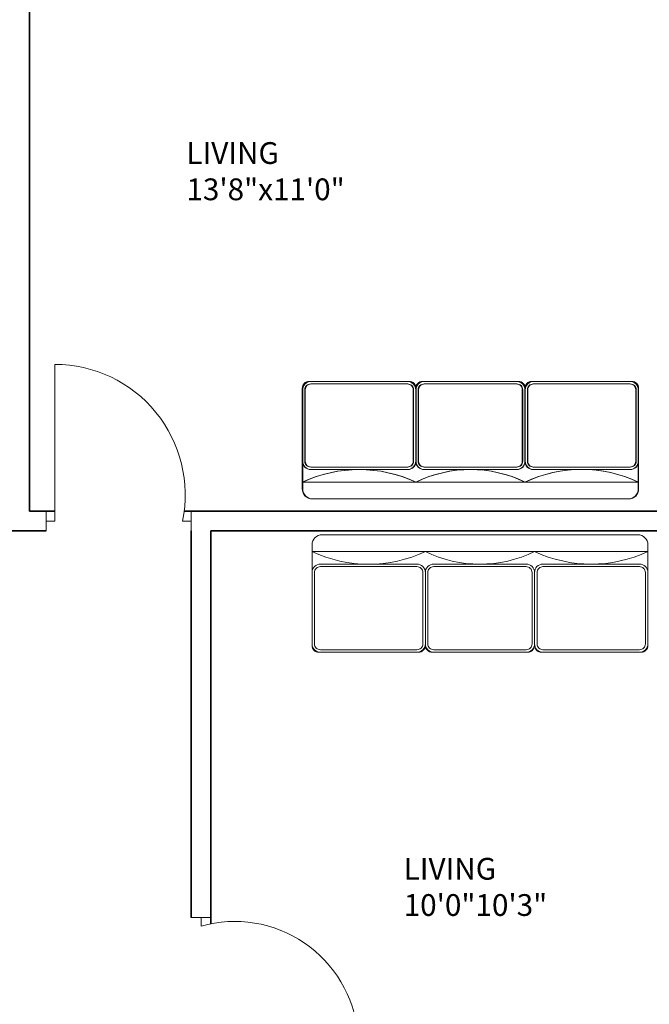
# Model space of a CAD drawing. Units: inches. Extents: x 2234 to 3001, y 1541 to 2386.
# Tile 8 of 12: x 2599 to 2744, y 1891 to 2118. Entities that reach past the tile are written whole.
import ezdxf

# ---------------------------------------------------------------- set-up
doc = ezdxf.new("R2010")
doc.units = ezdxf.units.IN
for name, color, linetype, lineweight in [('A-AREA-IDEN', 7, 'Continuous', 18), ('A-DOOR', 3, 'Continuous', 18), ('A-FURN', 9, 'Continuous', 13), ('A-WALL', 7, 'Continuous', 35)]:
    doc.layers.add(name, color=color, linetype=linetype, lineweight=lineweight)
doc.styles.get("Standard").update_dxf_attribs({"font": 'arial.ttf'})

# ---------------------------------------------------------------- blocks, each defined once
blk = doc.blocks.new('SOFA-3-SEAT')
for points in [[(1.93, 51.12), (18.33, 51.12, 0.414214), (20.26, 53.05), (20.26, 75.24, 0.414214), (18.33, 77.16), (1.93, 77.16, 0.414214), (0, 75.24), (0, 53.05, 0.414214)], [(1.93, 51.7), (18.33, 51.7, 0.414214), (19.68, 53.05), (19.68, 75.24, 0.414214), (18.33, 76.59), (1.93, 76.59, 0.414214), (0.58, 75.24), (0.58, 53.05, 0.414214)], [(1.93, 51.12), (18.33, 51.12, -0.414214), (20.26, 49.19), (20.26, 27.97, -0.414214), (18.33, 26.04), (1.93, 26.04, -0.414214), (0, 27.97), (0, 49.19, -0.414214)], [(1.93, 50.54), (18.33, 50.54, -0.414214), (19.68, 49.19), (19.68, 27.97, -0.414214), (18.33, 26.62), (1.93, 26.62, -0.414214), (0.58, 27.97), (0.58, 49.19, -0.414214)], [(1.93, 0), (18.33, 0, 0.414214), (20.26, 1.93), (20.26, 24.11, 0.414214), (18.33, 26.04), (1.93, 26.04, 0.414214), (0, 24.11), (0, 1.93, 0.414214)], [(1.93, 0.58), (18.33, 0.58, 0.414214), (19.68, 1.93), (19.68, 24.11, 0.414214), (18.33, 25.46), (1.93, 25.46, 0.414214), (0.58, 24.11), (0.58, 1.93, 0.414214)]]:
    blk.add_lwpolyline(points, format="xyb", close=True)
at = {"ltscale": 0.03}
blk.add_lwpolyline([(0, 24.48), (0, 1.54, 0.414214), (1.54, 0), (24.69, 0, 0.414214), (27.01, 2.31), (27.01, 74.85, 0.414214), (24.69, 77.16), (1.54, 77.16, 0.414214), (0, 75.62), (0, 52.68, 0.414214), (1.54, 51.14, -1), (1.54, 51.1, 0.414214), (0, 49.56), (0, 27.61, 0.414214), (1.54, 26.06, -1), (1.54, 26.02, 0.414214)], format="xyb", close=True, dxfattribs=at)
blk.add_lwpolyline([(23.15, 0), (23.15, 77.16)])
for centre, radius, start, end in [((50.64, 64.14), 30.42, 154.6538, 205.3462), ((48.71, 38.58), 28.47, 153.869, 206.131), ((50.96, 13.02), 30.71, 154.9106, 205.0894)]:
    blk.add_arc(centre, radius, start, end)

msp = doc.modelspace()

# ---------------------------------------------------------------- linework, layer by layer
at = {"layer": 'A-DOOR'}
for p, q in [((2607.0604, 2002.361), (2607.0604, 2038.361)), ((2605.0604, 2004.611), (2605.0604, 2000.111)), ((2638.4141, 2004.611), (2638.4141, 2004.611)), ((2638.4141, 2004.611), (2638.4141, 2000.111)), ((2605.0604, 2000.111), (2605.0604, 2002.361)), ((2605.0604, 2002.361), (2607.0604, 2002.361)), ((2638.4141, 2002.361), (2636.4141, 2002.361)), ((2638.4141, 2000.111), (2638.4141, 2002.361)), ((2638.4141, 1911.322), (2642.9141, 1911.322)), ((2642.9141, 1911.322), (2640.6641, 1911.322)), ((2640.6641, 1911.322), (2640.6641, 1909.322))]:
    msp.add_line(p, q, dxfattribs=at)
for centre, radius, start, end in [((2607.0604, 2008.3938), 29.9672, 348.38617, 90), ((2648.3788, 1881.9579), 28.4308, 5.798117, 105.744641)]:
    msp.add_arc(centre, radius, start, end, dxfattribs=at)
at = {"layer": 'A-WALL'}
for p, q in [((2601.2534, 2145.611), (2601.2534, 2004.611)), ((2601.2534, 2004.611), (2607.0604, 2004.611)), ((2636.7879, 2004.611), (2759.2534, 2004.611)), ((2593.6832, 2000.111), (2605.0604, 2000.111)), ((2638.4141, 2000.111), (2638.4141, 1911.322)), ((2642.9141, 2000.111), (2759.2534, 2000.111)), ((2642.9141, 2000.111), (2642.9141, 2000.111)), ((2642.9141, 1909.8586), (2642.9141, 2000.111))]:
    msp.add_line(p, q, dxfattribs=at)

# ---------------------------------------------------------------- block references
at = {"layer": 'A-FURN'}
for p, rotation in [((2663.9269, 2034.4483), 270), ((2663.9269, 2034.4483), 270), ((2664.0279, 2034.4483), 270), ((2664.0279, 2034.4483), 270), ((2743.3129, 1972.2215), 90), ((2743.3129, 1972.2215), 90)]:
    msp.add_blockref('SOFA-3-SEAT', p, dxfattribs=dict(at, rotation=rotation))

# ---------------------------------------------------------------- texts
at = {"layer": 'A-AREA-IDEN', "char_height": 5, "attachment_point": 1}
for s, width, insert in [('LIVING\\P13\'8"x11\'0"', 102.763163, (2637.303, 2089.4016)), ('LIVING\\P10\'0"10\'3"', 237.459688, (2687.2139, 1924.9979))]:
    msp.add_mtext_dynamic_manual_height_columns(s, width=width, gutter_width=12.5, heights=[0], dxfattribs=dict(at, insert=insert))

doc.saveas('drawing.dxf')
